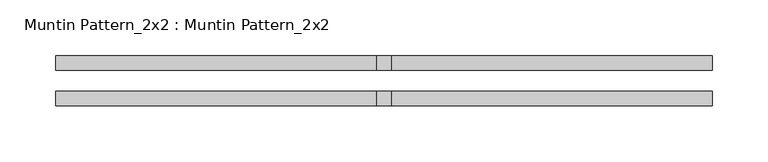
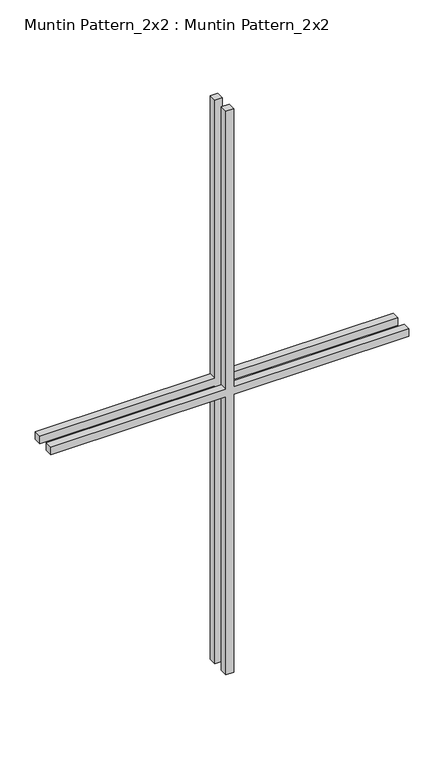
"""IFC4 building model written with IfcOpenShell, lengths in millimetres: proxy geometry, Muntin Pattern_2x2 : Muntin Pattern_2x2."""

from ifc_helpers import new_model, si_unit, frame, origin, place, context, project, spatial, polyline, outline, extrude, source, transform, mapped, element, save


def muntin_pattern_2x2_muntin_pattern_2x2_1fe271a4(model_context):
    return source(origin(), model_context, "Body", "SweptSolid", [
        extrude(outline(polyline([(495.3, -6.35), (495.3, -293.6875), (482.6, -293.6875), (482.6, -6.35), (0.0, -6.35), (0.0, 6.35), (482.6, 6.35), (482.6, 293.6875), (495.3, 293.6875), (495.3, 6.35), (977.9, 6.35), (977.9, -6.35), (495.3, -6.35)])), frame((0.0, 9.525, 0.0), z_axis=(0.0, 1.0, 0.0), x_axis=(0.0, 0.0, 1.0)), (0.0, 0.0, 1.0), 12.7),
        extrude(outline(polyline([(495.3, -6.35), (495.3, -293.6875), (482.6, -293.6875), (482.6, -6.35), (0.0, -6.35), (0.0, 6.35), (482.6, 6.35), (482.6, 293.6875), (495.3, 293.6875), (495.3, 6.35), (977.9, 6.35), (977.9, -6.35), (495.3, -6.35)])), frame((0.0, -22.225, 0.0), z_axis=(0.0, 1.0, 0.0), x_axis=(0.0, 0.0, 1.0)), (0.0, 0.0, 1.0), 12.7),
    ])


if __name__ == "__main__":
    model = new_model("IFC4")
    model_context = context("Model", 3, world=origin())
    ifc_project = project(units=[si_unit("LENGTHUNIT", "METRE", prefix="MILLI")], contexts=[model_context])
    site = spatial("IfcSite", under=ifc_project)
    building = spatial("IfcBuilding", under=site)
    placement = place(None, origin())
    muntin_pattern_2x2_muntin_pattern_2x2_shape = muntin_pattern_2x2_muntin_pattern_2x2_1fe271a4(model_context)
    element("IfcBuildingElementProxy", 1, Name="Muntin Pattern_2x2 : Muntin Pattern_2x2", ObjectType="Muntin Pattern_2x2 : Muntin Pattern_2x2", at=placement, inside=building, context=model_context, shape_type="MappedRepresentation", body=[
        mapped(muntin_pattern_2x2_muntin_pattern_2x2_shape, transform((0.0, 0.0, 0.0), x_axis=(1.0, 0.0, 0.0), y_axis=(0.0, 1.0, 0.0), z_axis=(0.0, 0.0, 1.0))),
    ])
    save(model, "model.ifc")

# Revit data of these elements
# Type "Muntin Pattern_2x2 : Muntin Pattern_2x2"
#   Width [instance default] = 48"
#   Thickness = 0.5"
#   Height [instance default] = 48"
#   Distance = 0.75"
#   Interior Material [instance default] = none
#   Exterior Material [instance default] = none
#   Default Elevation = 0
# Element 1 (IfcBuildingElementProxy, "Muntin Pattern_2x2 : Muntin Pattern_2x2")
#   Width = 23.125"
#   Height = 38.5"
#   Interior Material = Wood - Stained
#   Exterior Material = Clad - White
#   Materials on its faces: "Clad - White", "Wood - Stained"
# Materials
#   "Clad - White": class "Wood", colour RGB 242 242 238, transparency 0, Cost = 0
#   "Wood - Stained": class "Wood", colour RGB 224 178 126, transparency 0, Cost = 0
